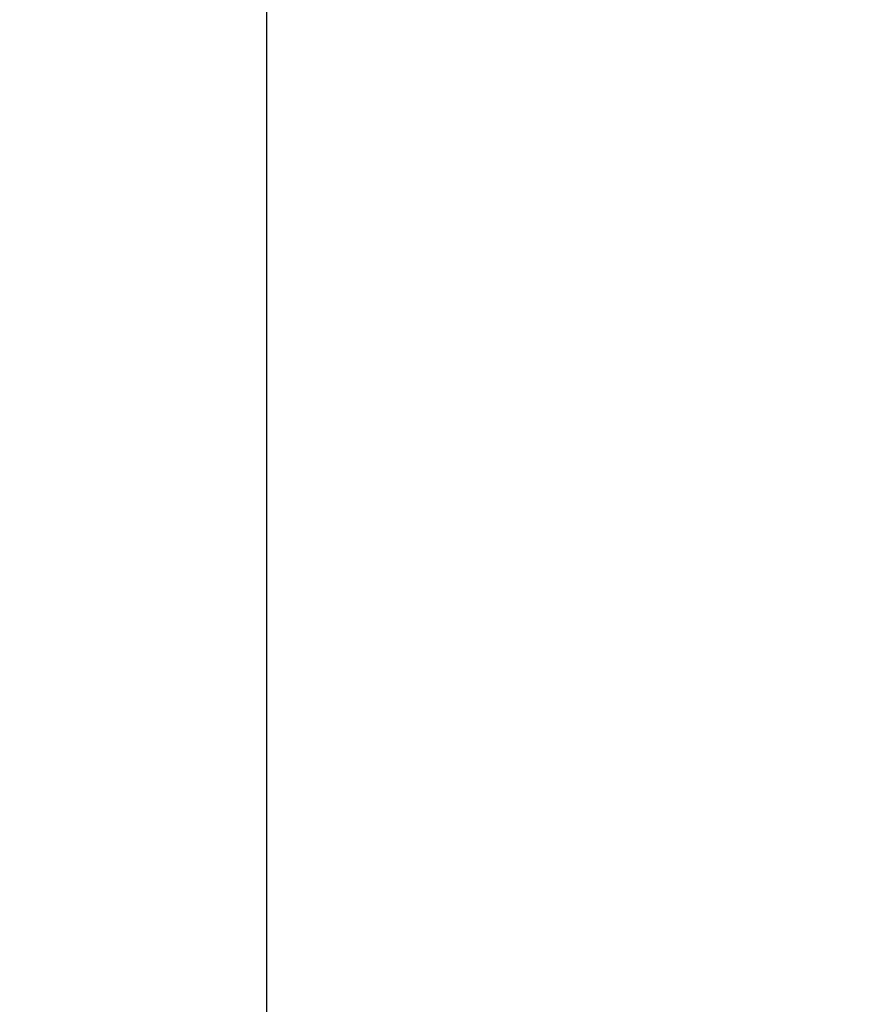
# Model space of a CAD drawing. Units: inches. Extents: x 2696 to 3240, y 1564 to 2310.
# Tile 7 of 76: x 2903.4 to 2912.11, y 1633.53 to 1643.56. Entities that reach past the tile are written whole.
import ezdxf

# ---------------------------------------------------------------- set-up
doc = ezdxf.new("R2010")
doc.units = ezdxf.units.IN
doc.layers.add('A-ANNO-DIMS', color=3, linetype='Continuous', lineweight=18)
doc.styles.add('TIMES NEW', font='times.ttf')
doc.dimstyles.new('Siddhuu', dxfattribs={"dimtxt": 6, "dimasz": 2.5, "dimexe": 1.25, "dimexo": 0.625, "dimtad": 1, "dimdec": 1, "dimlunit": 4, "dimtxsty": 'TIMES NEW', "dimcen": 2.5, "dimclrd": 256, "dimclre": 1, "dimclrt": 7, "dimadec": 0, "dimazin": 0, "dimtfac": 1, "dimtdec": 1, "dimtmove": 0, "dimatfit": 3, "dimfxl": 1, "dimtolj": 1, "dimlwd": -1, "dimarcsym": 0})

# ---------------------------------------------------------------- blocks, each defined once
blk = doc.blocks.new('*D36')
at = {"layer": 'A-ANNO-DIMS', "color": 1, "lineweight": -2, "transparency": 16777216}
for p, q in [((3008.237, 1629.386), (3008.237, 1619.461)), ((3070.237, 1629.386), (3070.237, 1619.461))]:
    blk.add_line(p, q, dxfattribs=at)
at = {"layer": 'A-ANNO-DIMS', "transparency": 16777216}
for p, q in [((3008.237, 1620.711), (2894.718, 1620.711)), ((3067.737, 1620.711), (3010.737, 1620.711))]:
    blk.add_line(p, q, dxfattribs=at)
for points in [[(3010.737, 1621.128), (3010.737, 1620.294), (3008.237, 1620.711)], [(3067.737, 1621.128), (3067.737, 1620.294), (3070.237, 1620.711)]]:
    blk.add_solid(points, dxfattribs=at)
at = {"layer": 'Defpoints', "color": 0, "transparency": 16777216}
for p in [(3008.237, 1630.011), (3070.237, 1630.011), (3008.237, 1620.711)]:
    blk.add_point(p, dxfattribs=at)
at = {"layer": 'A-ANNO-DIMS', "color": 7, "transparency": 16777216, "insert": (2950.228, 1624.403), "char_height": 6, "attachment_point": 5, "style": 'TIMES NEW'}
blk.add_mtext('\\A1;BALCONY DOOR 5\'-2" TYP.', dxfattribs=at)
blk = doc.blocks.new('*D57')
at = {"layer": 'A-ANNO-DIMS', "color": 1, "lineweight": -2, "transparency": 16777216}
for p, q in [((2754.611, 2018.576), (2754.611, 1568.951)), ((2956.709, 2018.576), (2956.709, 1568.951))]:
    blk.add_line(p, q, dxfattribs=at)
at = {"layer": 'A-ANNO-DIMS', "transparency": 16777216}
blk.add_line((2757.111, 1570.201), (2954.209, 1570.201), dxfattribs=at)
for points in [[(2757.111, 1570.618), (2757.111, 1569.784), (2754.611, 1570.201)], [(2954.209, 1570.618), (2954.209, 1569.784), (2956.709, 1570.201)]]:
    blk.add_solid(points, dxfattribs=at)
at = {"layer": 'Defpoints', "color": 0, "transparency": 16777216}
for p in [(2754.611, 2019.201), (2956.709, 2019.201), (2956.709, 1570.201)]:
    blk.add_point(p, dxfattribs=at)
at = {"layer": 'A-ANNO-DIMS', "color": 7, "transparency": 16777216, "insert": (2855.66, 1573.878), "char_height": 6, "attachment_point": 5, "style": 'TIMES NEW'}
blk.add_mtext('\\A1;16\'-10"', dxfattribs=at)
blk = doc.blocks.new('*D69')
at = {"layer": 'A-ANNO-DIMS', "color": 1, "lineweight": -2, "transparency": 16777216}
for p, q in [((2841.889, 2261.576), (2841.889, 1568.951)), ((2905.91, 2261.576), (2905.91, 1568.951))]:
    blk.add_line(p, q, dxfattribs=at)
at = {"layer": 'A-ANNO-DIMS', "transparency": 16777216}
blk.add_line((2844.389, 1570.201), (2903.41, 1570.201), dxfattribs=at)
for points in [[(2844.389, 1570.618), (2844.389, 1569.784), (2841.889, 1570.201)], [(2903.41, 1570.618), (2903.41, 1569.784), (2905.91, 1570.201)]]:
    blk.add_solid(points, dxfattribs=at)
at = {"layer": 'Defpoints', "color": 0, "transparency": 16777216}
for p in [(2841.889, 2262.201), (2905.91, 2262.201), (2905.91, 1570.201)]:
    blk.add_point(p, dxfattribs=at)
at = {"layer": 'A-ANNO-DIMS', "color": 7, "transparency": 16777216, "insert": (2873.9, 1573.878), "char_height": 6, "attachment_point": 5, "style": 'TIMES NEW'}
blk.add_mtext('\\A1;5\'-4"', dxfattribs=at)

msp = doc.modelspace()

# ---------------------------------------------------------------- dimensions: what is measured, and where the dimension line sits
at = {"layer": 'A-ANNO-DIMS'}
for base, p1, p2, picture, middle in [((2905.91, 1570.201), (2841.889, 2262.201), (2905.91, 2262.201), '*D69', (2873.9, 1573.878)), ((2956.709, 1570.201), (2754.611, 2019.201), (2956.709, 2019.201), '*D57', (2855.66, 1573.878))]:
    dim = msp.add_linear_dim(base=base, p1=p1, p2=p2, dimstyle='Siddhuu', override={"dimdec": 1, "dimlfac": 1, "dimrnd": 0, "dimzin": 1, "dimdsep": 46, "dimlunit": 4, "dimfrac": 2}, dxfattribs=at)
    dim.commit()
    dim.dimension.update_dxf_attribs({"geometry": picture, "text_midpoint": middle})
dim = msp.add_linear_dim(base=(3008.237, 1620.711), p1=(3070.237, 1630.011), p2=(3008.237, 1630.011), angle=180, text='BALCONY DOOR <> TYP.', dimstyle='Siddhuu', override={"dimdec": 1, "dimlfac": 1, "dimrnd": 0, "dimzin": 1, "dimdsep": 46, "dimlunit": 4, "dimfrac": 2}, dxfattribs=at)
dim.commit()
dim.dimension.update_dxf_attribs({"geometry": '*D36', "text_midpoint": (2950.228, 1624.403)})

doc.saveas('drawing.dxf')
